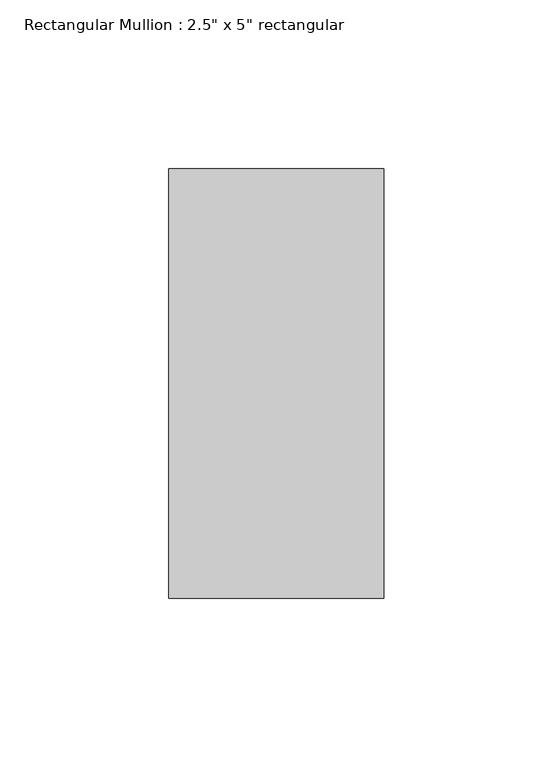
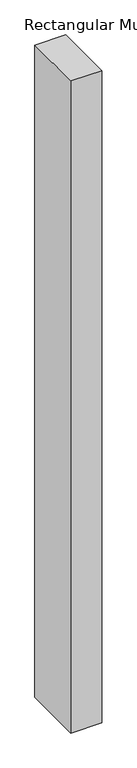
"""IFC4 building model written with IfcOpenShell, lengths in millimetres: member geometry."""

from ifc_helpers import new_model, si_unit, frame, origin, place, context, project, spatial, polyline, outline, extrude, source, transform, mapped, element, save


def member_4c43c051(model_context):
    return source(origin(), model_context, "Body", "SweptSolid", [
        extrude(outline(polyline([(31.75, 63.5), (31.75, -63.5), (-31.75, -63.5), (-31.75, 63.5), (31.75, 63.5)])), frame((0.0, 0.0, -1410.3945466), z_axis=(0.0, 0.0, 1.0), x_axis=(1.0, 0.0, 0.0)), (0.0, 0.0, 1.0), 1410.3945466),
    ])


if __name__ == "__main__":
    model = new_model("IFC4")
    model_context = context("Model", 3, world=origin())
    ifc_project = project(units=[si_unit("LENGTHUNIT", "METRE", prefix="MILLI")], contexts=[model_context])
    site = spatial("IfcSite", under=ifc_project)
    building = spatial("IfcBuilding", under=site)
    placement = place(None, origin())
    member_shape = member_4c43c051(model_context)
    element("IfcMember", 1, ObjectType="Rectangular Mullion : 2.5\" x 5\" rectangular", at=placement, inside=building, context=model_context, shape_type="MappedRepresentation", body=[
        mapped(member_shape, transform((0.0, 0.0, 0.0), x_axis=(1.0, 0.0, 0.0), y_axis=(0.0, 1.0, 0.0), z_axis=(0.0, 0.0, 1.0))),
    ])
    save(model, "model.ifc")

# Revit data of these elements
# Type "Rectangular Mullion : 2.5\" x 5\" rectangular"
#   built-in parameter 1007304 = 0.416667 (stored number, unit not read)
#   built-in parameter 1007301 = 0.104167 (stored number, unit not read)
#   built-in parameter 1007300 = 0.104167 (stored number, unit not read)
# Element 1 (IfcMember, "Rectangular Mullion : 2.5\" x 5\" rectangular")
#   Materials on its faces: "Aluminum"
# Materials
#   "Aluminum": class "Metal", colour RGB 247 247 247, transparency 0, Description = "Aluminum 6061", Cost = 0
